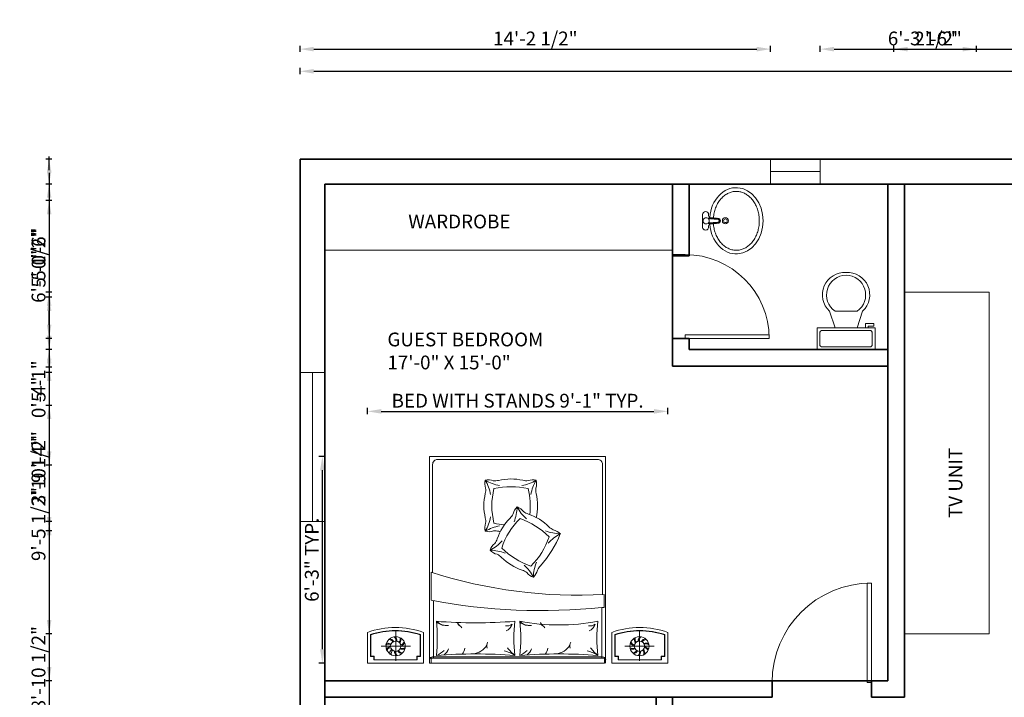
# Model space of a CAD drawing. Units: inches. Extents: x -100 to 766, y -562 to 63.
# Tile 8 of 11: x -100 to 257, y -182 to 63. Entities that reach past the tile are written whole.
import ezdxf

# ---------------------------------------------------------------- set-up
doc = ezdxf.new("R2010")
doc.units = ezdxf.units.IN
for name, color, linetype, lineweight in [('A-ANNO-DIMS', 2, 'Continuous', 18), ('A-ANNO-TEXT', 7, 'Continuous', 18), ('A-AREA-IDEN', 7, 'Continuous', 18), ('A-DOOR', 3, 'Continuous', 18), ('A-FLOR-CASE', 32, 'Continuous', 18), ('A-FLOR-FIXT', 8, 'Continuous', 18), ('A-GLAZ', 4, 'Continuous', 18), ('A-WALL', 7, 'Continuous', 35), ('furn', 8, 'Continuous', 13)]:
    doc.layers.add(name, color=color, linetype=linetype, lineweight=lineweight)
doc.styles.get("Standard").update_dxf_attribs({"font": 'arial.ttf'})
doc.dimstyles.new('ISO-25', dxfattribs={"dimtxt": 5, "dimasz": 5, "dimexe": 1.25, "dimexo": 0.625, "dimtad": 1, "dimlunit": 3, "dimtxsty": 'Standard', "dimcen": 2.5, "dimadec": 0, "dimazin": 0, "dimtfac": 1, "dimtmove": 0, "dimatfit": 3, "dimfxl": 1, "dimfxlon": 1, "dimarcsym": 0})

# ---------------------------------------------------------------- blocks, each defined once
blk = doc.blocks.new('*U2')
for p, q in [((0, 0), (0, -6)), ((40, 0), (40, -6))]:
    blk.add_line(p, q)
blk.add_lwpolyline([(0, 0), (0, 40), (1.75, 40), (1.75, 0)], close=True)
blk.add_arc((0, 0), 40, 0, 90)
blk = doc.blocks.new('*U4')
for p, q in [((9.5, -6), (9.5, -2)), ((-10, -8.5), (-8, -8.5)), ((-10, -9.5), (-10, -8.5)), ((-7, -9.5), (-10, -9.5)), ((-8, -8.5), (-8, -8)), ((-7, -8), (-7, -9.5)), ((-4, -8), (-6, -14)), ((4, -8), (6, -14)), ((4, -14), (-4, -14))]:
    blk.add_line(p, q)
blk.add_lwpolyline([(10.5, -8), (10.5, 0), (-10.5, 0), (-10.5, -8)], close=True)
for points in [[(-9.5, -2), (-9.5, -6)], [(8.5, -1), (-8.5, -1)], [(-8.5, -7), (8.5, -7)]]:
    blk.add_lwpolyline(points)
for centre, radius, start, end in [((-8.625, -1.875), 0.8839, 81.8699, 188.1301), ((8.625, -1.875), 0.8839, 351.8699, 98.1301), ((-8.625, -6.125), 0.8839, 171.869898, 278.1301), ((8.625, -6.125), 0.8839, 261.8699, 8.1301), ((-0.4772, -19.9188), 8.0953, 133.01722, 273.38), ((0.0374, -19.8731), 7.127, 124.50543, 269.7), ((-0.0373, -19.8731), 7.127, 270.3, 55.4946), ((0.4773, -19.9188), 8.0953, 266.62, 46.9828)]:
    blk.add_arc(centre, radius, start, end)
blk = doc.blocks.new('*D9')
at = {"layer": 'A-ANNO-DIMS', "color": 0, "lineweight": -2, "transparency": 16777216}
for p, q in [((1.39, 43.65), (1.39, 45.9)), ((6.39, 44.65), (716.39, 44.65)), ((721.39, 43.65), (721.39, 45.9))]:
    blk.add_line(p, q, dxfattribs=at)
at = {"layer": 'A-ANNO-DIMS', "color": 0, "transparency": 16777216}
for points in [[(6.39, 45.48), (6.39, 43.82), (1.39, 44.65)], [(716.39, 45.48), (716.39, 43.82), (721.39, 44.65)]]:
    blk.add_solid(points, dxfattribs=at)
at = {"layer": 'Defpoints', "color": 0, "transparency": 16777216}
for p in [(721.39, 44.65), (1.39, 12.79), (721.39, 12.79)]:
    blk.add_point(p, dxfattribs=at)
at = {"layer": 'A-ANNO-DIMS', "color": 0, "transparency": 16777216, "insert": (361.39, 47.83), "char_height": 5, "attachment_point": 5}
blk.add_mtext("60'", dxfattribs=at)
blk = doc.blocks.new('A$C359865C9')
for p, q in [((0.26, 0.5858), (0.38, 0.5858)), ((0.26, 0.5258), (0.272, 0.5258)), ((0.368, 0.5258), (0.3809, 0.5258))]:
    blk.add_line(p, q)
for radius in [0.03, 0.018]:
    blk.add_circle((0.3201, 0.3632), radius)
for centre, radius, start, end in [((0.26, 0.5558), 0.03, 90.00613, 270.00613), ((0.32, 0.5495), 0.03, 348.15369, 191.84631), ((0.38, 0.5558), 0.03, 270.00613, 89.98161), ((0.272, 0.5078), 0.018, 0.00613, 90.00613), ((0.32, 0.5495), 0.03, 222.45226, 317.54774), ((0.368, 0.5078), 0.018, 90.00613, 180.00613), ((0.3201, 0.4358), 0.024, 180.00613, 0.00613), ((0.3201, 0.4358), 0.0204, 180.00613, 0.00613), ((0.3201, 0.4358), 0.0144, 180.00613, 0.00613)]:
    blk.add_arc(centre, radius, start, end)
at = {"extrusion": (0, 0, -1)}
blk.add_ellipse((0.3199, 0.5826), major_axis=(-0.00812, 0), ratio=0.392595, dxfattribs=at)
at = {"ltscale": 100, "extrusion": (0, 0, -1)}
blk.add_ellipse((0.3201, 0.258), major_axis=(0.3216, 0), ratio=0.80597, start_param=-1.471508, end_param=4.612925, dxfattribs=at)
for points, knots in [([(0.3475, 0.4801), (0.3477, 0.4801), (0.3479, 0.4801), (0.3648, 0.4788), (0.3813, 0.4763), (0.4136, 0.4692), (0.4293, 0.4645), (0.4593, 0.4531), (0.4737, 0.4464), (0.5006, 0.4312), (0.5131, 0.4227), (0.5361, 0.4042), (0.5465, 0.3942), (0.5649, 0.3732), (0.5729, 0.3622), (0.5864, 0.3393), (0.5918, 0.3275), (0.6, 0.3036), (0.6029, 0.2914), (0.6059, 0.2669), (0.6061, 0.2545), (0.6039, 0.2301), (0.6015, 0.218), (0.5941, 0.1942), (0.5892, 0.1825), (0.5768, 0.1597), (0.5693, 0.1486), (0.552, 0.1275), (0.5422, 0.1174), (0.5203, 0.0986), (0.5083, 0.0899), (0.4825, 0.0741), (0.4686, 0.0671), (0.4396, 0.0549), (0.4243, 0.0498), (0.3929, 0.0418), (0.3767, 0.0388), (0.3439, 0.0352), (0.3273, 0.0344), (0.2942, 0.0353), (0.2776, 0.0369), (0.2452, 0.0422), (0.2293, 0.046), (0.1987, 0.0556), (0.1839, 0.0615), (0.156, 0.0751), (0.1428, 0.0828), (0.1184, 0.0997), (0.1071, 0.109), (0.0869, 0.1288), (0.078, 0.1393), (0.0625, 0.1611), (0.0559, 0.1725), (0.0454, 0.1957), (0.0415, 0.2076), (0.036, 0.2317), (0.0346, 0.2438), (0.0345, 0.2566), (0.0345, 0.2573), (0.0345, 0.258), (0.0345, 0.2664), (0.0351, 0.2749), (0.0382, 0.2956), (0.0413, 0.3078), (0.0502, 0.3317), (0.0559, 0.3434), (0.0699, 0.3661), (0.0782, 0.377), (0.0972, 0.3978), (0.1079, 0.4076), (0.1313, 0.4257), (0.1441, 0.434), (0.1714, 0.4488), (0.186, 0.4553), (0.2163, 0.4662), (0.2321, 0.4706), (0.2628, 0.4769), (0.2776, 0.479), (0.2925, 0.4801)], [1.664851, 1.664851, 1.664851, 1.664851, 1.666804, 1.666804, 1.838807, 1.838807, 2.01081, 2.01081, 2.182814, 2.182814, 2.354817, 2.354817, 2.52682, 2.52682, 2.698824, 2.698824, 2.870827, 2.870827, 3.04283, 3.04283, 3.214834, 3.214834, 3.384783, 3.384783, 3.554732, 3.554732, 3.724681, 3.724681, 3.89463, 3.89463, 4.064578, 4.064578, 4.234527, 4.234527, 4.404476, 4.404476, 4.574425, 4.574425, 4.744374, 4.744374, 4.914323, 4.914323, 5.084272, 5.084272, 5.254221, 5.254221, 5.42417, 5.42417, 5.594119, 5.594119, 5.764068, 5.764068, 5.934016, 5.934016, 6.103965, 6.103965, 6.273914, 6.273914, 6.283185, 6.283185, 6.283185, 6.401959, 6.401959, 6.573962, 6.573962, 6.745965, 6.745965, 6.917969, 6.917969, 7.089972, 7.089972, 7.261975, 7.261975, 7.433979, 7.433979, 7.605982, 7.605982, 7.759676, 7.759676, 7.759676, 7.759676]), ([(0.29, 0.5078), (0.2913, 0.4937), (0.2935, 0.4697), (0.2953, 0.4457), (0.2961, 0.4358)], [0, 0, 0, 0, 35.358253, 60.208758, 60.208758, 60.208758, 60.208758]), ([(0.2907, 0.5434), (0.2946, 0.498), (0.2952, 0.4908), (0.2965, 0.4761), (0.2971, 0.4686), (0.2983, 0.4536), (0.2989, 0.4461), (0.2995, 0.4378), (0.2996, 0.4369), (0.2996, 0.4361)], [2.511178, 2.511178, 2.511178, 2.511178, 20.495008, 20.495008, 39.297594, 39.297594, 58.10018, 58.10018, 60.208758, 60.208758, 60.208758, 60.208758]), ([(0.2979, 0.5293), (0.298, 0.528), (0.2981, 0.5267), (0.2988, 0.5184), (0.2993, 0.5127), (0.3005, 0.4986), (0.301, 0.4933), (0.3014, 0.4884), (0.3015, 0.4875), (0.3017, 0.4857), (0.3017, 0.485), (0.3019, 0.4827), (0.3021, 0.4812), (0.3026, 0.4756), (0.3029, 0.4716), (0.3037, 0.4621), (0.3041, 0.4568), (0.3049, 0.4464), (0.3053, 0.4415), (0.3056, 0.4365)], [4.643985, 4.643985, 4.643985, 4.643985, 5.282102, 5.282102, 8.976667, 8.976667, 16.365798, 16.365798, 18.536065, 18.536065, 20.434607, 20.434607, 24.231692, 24.231692, 34.371999, 34.371999, 47.807513, 47.807513, 60.208758, 60.208758, 60.208758, 60.208758]), ([(0.3422, 0.5293), (0.3421, 0.528), (0.342, 0.5267), (0.3412, 0.5184), (0.3408, 0.5127), (0.3395, 0.4986), (0.3391, 0.4933), (0.3387, 0.4884), (0.3386, 0.4875), (0.3384, 0.4857), (0.3383, 0.485), (0.3381, 0.4827), (0.338, 0.4812), (0.3375, 0.4756), (0.3372, 0.4716), (0.3364, 0.4621), (0.336, 0.4568), (0.3352, 0.4464), (0.3348, 0.4415), (0.3345, 0.4365)], [4.643985, 4.643985, 4.643985, 4.643985, 5.282102, 5.282102, 8.976667, 8.976667, 16.365798, 16.365798, 18.536065, 18.536065, 20.434607, 20.434607, 24.231692, 24.231692, 34.371999, 34.371999, 47.807513, 47.807513, 60.208758, 60.208758, 60.208758, 60.208758]), ([(0.3494, 0.5434), (0.3455, 0.498), (0.3449, 0.4908), (0.3436, 0.4761), (0.343, 0.4686), (0.3418, 0.4536), (0.3412, 0.4461), (0.3406, 0.4378), (0.3405, 0.4369), (0.3404, 0.4361)], [2.511178, 2.511178, 2.511178, 2.511178, 20.495008, 20.495008, 39.297594, 39.297594, 58.10018, 58.10018, 60.208758, 60.208758, 60.208758, 60.208758]), ([(0.35, 0.5078), (0.3487, 0.4937), (0.3466, 0.4697), (0.3448, 0.4457), (0.344, 0.4358)], [0, 0, 0, 0, 35.358253, 60.208758, 60.208758, 60.208758, 60.208758])]:
    blk.add_open_spline(points, degree=3, knots=knots)
blk = doc.blocks.new('WIN-54IN')
blk.add_line((4.5, 54), (4.5, 0))
blk.add_lwpolyline([(0, 54), (9, 54), (9, 0), (0, 0)], close=True)
blk = doc.blocks.new('WIN-18IN')
blk.add_line((4.5, 18), (4.5, 0))
blk.add_lwpolyline([(0, 18), (9, 18), (9, 0), (0, 0)], close=True)
blk = doc.blocks.new('BED-DOUBLE-WITH-NIGHTSTANDS')
for p, q in [((23.96, 1.73), (23.96, 22.55)), ((84.9, 1.73), (84.9, 20.16)), ((10.25, 11.43), (10.25, 0.8)), ((98.58, 11.43), (98.58, 0.79)), ((4.93, 6.11), (15.57, 6.11)), ((103.9, 6.11), (93.26, 6.11)), ((85.22, 2.28), (23.61, 2.28))]:
    blk.add_line(p, q)
for points in [[(86.32, 0), (86.32, 74.89), (22.5, 74.89), (22.5, 0)], [(2.43, 1.11), (2.43, 2.44), (1.11, 2.44)], [(2.32, 1.11), (2.32, 2.32), (1.11, 2.32)], [(2.32, 1.22), (17.97, 1.22)], [(2.32, 1.11), (17.97, 1.11)], [(17.85, 1.11), (17.85, 2.44), (19.18, 2.44)], [(17.97, 1.11), (17.97, 2.32), (19.18, 2.32)], [(23.1, 0), (23.1, 1.73), (85.95, 1.73), (85.95, 0), (22.5, 0)], [(90.97, 1.11), (90.97, 2.44), (89.64, 2.44)], [(90.86, 1.11), (90.86, 2.33), (89.64, 2.33)], [(106.5, 1.22), (90.86, 1.22)], [(106.5, 1.11), (90.86, 1.11)], [(106.39, 1.11), (106.39, 2.44), (107.72, 2.44)], [(106.5, 1.11), (106.5, 2.33), (107.72, 2.33)]]:
    blk.add_lwpolyline(points)
for points in [[(85.22, 24.82), (85.22, 71.94, 0.414214), (83.37, 73.78), (25.45, 73.78, 0.414214), (23.61, 71.94), (23.61, 32.78)], [(42.71, 66.24, 0.159461), (42.84, 63.34, -0.076283), (42.71, 61.4, 0.115075), (42.71, 52.64, -0.076283), (42.84, 50.7, 0.159461), (42.71, 47.8)], [(44.62, 61.06, 0.091296), (42.71, 66.24, 0.091296), (47.89, 64.35)], [(55.97, 64.35, 0.091296), (61.15, 66.24, 0.091296), (59.25, 61.06, 0.091296)], [(58.24, 63.23, 0.111006), (45.84, 63.22, 0.119549), (45.84, 50.66, 0.033212), (49.65, 50.08)], [(54.24, 56.57, 0.159461), (52.81, 54.04, -0.076283), (51.68, 52.46, 0.115075), (47.05, 45.03, -0.076283), (46.13, 43.32, 0.159461), (44.49, 40.92)], [(53.12, 51.17, 0.091296), (54.24, 56.57, 0.091296), (57.64, 52.23)], [(47.89, 49.69, 0.091296), (42.71, 47.8, 0.091296), (44.62, 52.98, 0.091296)], [(65.83, 45.8, 0.111006), (55.29, 52.35, 0.119549), (48.65, 41.69, 0.107813), (59.16, 35.11)], [(64.49, 47.96, 0.091296), (69.89, 46.82, 0.091296), (65.54, 43.43, 0.091296)], [(49.89, 39.78, 0.091296), (44.49, 40.92, 0.091296), (48.84, 44.31, 0.091296)], [(59.21, 35.12, 0.121865), (65.83, 45.8, 0.121865)], [(61.26, 36.57, 0.091296), (60.14, 31.16, 0.091296), (56.74, 35.51, 0.091296)], [(19.18, 2.32), (19.18, 10.3, 0.167087), (1.11, 10.3), (1.11, 2.32)], [(19.07, 2.32), (19.07, 10.22, 0.165559), (1.22, 10.22), (1.22, 2.32)], [(89.64, 2.33), (89.64, 10.3, -0.167087), (107.72, 10.3), (107.72, 2.33)], [(89.75, 2.33), (89.75, 10.22, -0.165559), (107.61, 10.22), (107.61, 2.33)]]:
    blk.add_lwpolyline(points, format="xyb")
for points in [[(85.77, 20.16), (84.9, 20.16, -0.072944), (23.1, 22.73), (23.1, 32.96, 0.092568), (85.77, 24.85)], [(53.41, 15.12, 0.058596), (53.41, 2.79, 0.036648), (24.98, 2.79, 0.052163), (24.98, 15.12, 0.036967)], [(83.49, 15.12, 0.058596), (83.49, 2.79, 0.036889), (55.25, 2.79, 0.052163), (55.25, 15.12, 0.093111)], [(0, 11.07), (0, 0), (20.29, 0), (20.29, 11.07, 0.181818)], [(108.83, 11.07), (108.83, 0), (88.54, 0), (88.54, 11.07, -0.181818)]]:
    blk.add_lwpolyline(points, format="xyb", close=True)
for centre, radius in [((10.25, 6.11), 3.48), ((10.25, 6.11), 1.88), ((98.58, 6.11), 3.48), ((98.58, 6.11), 1.88)]:
    blk.add_circle(centre, radius)
for centre, radius, start, end in [((43.85, 61.01), 5.35, 70.7023, 102.284), ((46.15, 72.45), 6.4, 265.2252, 282.6741), ((51.99, 47.44), 19.27, 77.0576, 103.3153), ((57.67, 72.48), 6.4, 257.6988, 275.1477), ((59.91, 61.73), 4.68, 74.5791, 110.8198), ((56.65, 64.98), 4.68, 339.3666, 15.6073), ((32.87, 56.89), 26.15, 353.1956, 14.0284), ((67.41, 62.78), 6.4, 175.0387, 192.4877), ((42.38, 57.02), 19.27, 346.8711, 13.1289), ((52.44, 51.53), 5.35, 38.7754, 70.3571), ((60.44, 60.02), 6.4, 233.2983, 250.7472), ((52.18, 35.71), 19.27, 45.1307, 71.3884), ((44.09, 51.89), 4.32, 251.3996, 291.5774), ((46.25, 41.5), 6.4, 77.6988, 95.1477), ((51.93, 66.54), 19.27, 257.0576, 258.7033), ((32.5, 62.1), 40.4, 318.3818, 337.7644), ((70.24, 53.96), 6.4, 225.7718, 243.2208), ((66.46, 43.65), 4.68, 42.6522, 78.8929), ((47.82, 43.66), 4.32, 219.4726, 259.6505), ((44.16, 33.7), 6.4, 45.7718, 63.2208), ((62.22, 51.95), 19.27, 225.1307, 251.3884), ((53.96, 27.63), 6.4, 53.2983, 70.7472), ((61.38, 35.5), 4.51, 217.2937, 254.0973), ((56.98, 34.61), 4.68, 312.4658, 348.7065), ((67.28, 30.79), 6.4, 135.5854, 153.0343), ((27.82, 16.88), 3.19, 213.6349, 270.8456), ((28.76, 18.64), 5.04, 224.406, 276.8342), ((33.7, 14.59), 1.03, 173.7543, 257.2187), ((45.1, 23.69), 15.4, 216.2085, 225.0849), ((58.85, 18.64), 5.04, 224.406, 276.8342), ((57.9, 16.88), 3.19, 213.6349, 270.8456), ((63.79, 14.59), 1.03, 173.7543, 257.2187), ((75.18, 23.69), 15.4, 216.2085, 225.0849), ((50.68, 16.26), 2.8, 256.4823, 308.5563), ((48.55, 15.4), 4.1, 294.2916, 340.9896), ((80.77, 16.26), 2.8, 256.4823, 308.5563), ((78.64, 15.4), 4.1, 294.2916, 340.9896), ((7.62, 4.92), 2.23, 69.5103, 115.83), ((7.79, 6.82), 1.7, 31.462, 91.6998), ((7.68, 6.63), 2.23, 33.5103, 79.83), ((8.68, 8.13), 1.7, 355.462, 55.6998), ((8.47, 8.04), 2.23, 357.5103, 43.83), ((10.16, 8.67), 1.7, 319.462, 19.6998), ((9.94, 8.72), 2.23, 321.5103, 7.83), ((11.68, 8.23), 1.7, 283.462, 343.6998), ((11.53, 8.4), 2.23, 285.5103, 331.83), ((46.36, 6.29), 3.06, 155.8927, 196.1192), ((76.44, 6.29), 3.06, 155.8927, 196.1192), ((97.3, 8.4), 2.23, 208.17, 254.4897), ((97.15, 8.23), 1.7, 196.3002, 256.538), ((98.88, 8.72), 2.23, 172.17, 218.4897), ((98.67, 8.67), 1.7, 160.3002, 220.538), ((100.36, 8.04), 2.23, 136.17, 182.4897), ((100.15, 8.13), 1.7, 124.3002, 184.538), ((101.15, 6.63), 2.23, 100.17, 146.4897), ((101.03, 6.82), 1.7, 88.3002, 148.538), ((100.96, 5.02), 2.23, 64.17, 110.4897), ((7.59, 5.14), 1.7, 67.462, 127.6998), ((8.72, 3.73), 2.23, 105.5103, 151.83), ((8.57, 3.9), 1.7, 103.462, 163.6998), ((10.3, 3.42), 2.23, 141.5103, 187.83), ((10.34, 3.56), 1.7, 139.462, 199.6998), ((12.03, 4.19), 2.23, 177.5103, 223.83), ((11.82, 4.1), 1.7, 175.462, 235.6998), ((12.82, 5.6), 2.23, 213.5103, 259.83), ((12.71, 5.41), 1.7, 211.462, 271.6998), ((12.63, 7.21), 2.23, 249.5103, 295.83), ((12.65, 6.99), 1.7, 247.462, 307.6998), ((21.28, 11.24), 9.3, 294.6457, 314.1585), ((24.5, 6.89), 5.16, 310.5354, 340.3558), ((30.57, 6.21), 4.8, 321.8174, 349.8987), ((37.48, 10.1), 6.84, 276.6849, 328.3182), ((46.85, -7.52), 12.22, 57.5379, 77.5233), ((62.65, 14.32), 14.78, 216.4935, 231.2792), ((51.37, 11.24), 9.3, 294.6457, 314.1585), ((54.59, 6.89), 5.16, 310.5354, 340.3558), ((60.65, 6.21), 4.8, 321.8174, 349.8987), ((67.57, 10.1), 6.84, 276.6849, 328.3182), ((76.94, -7.52), 12.22, 57.5379, 77.5233), ((92.74, 14.32), 14.78, 216.4935, 231.2792), ((96.17, 6.99), 1.7, 232.3002, 292.538), ((96.2, 7.21), 2.23, 244.17, 290.4897), ((96.12, 5.41), 1.7, 268.3002, 328.538), ((96.01, 5.6), 2.23, 280.17, 326.4897), ((97, 4.1), 1.7, 304.3002, 4.538), ((96.8, 4.19), 2.23, 316.17, 2.4897), ((98.49, 3.56), 1.7, 340.3002, 40.538), ((98.27, 3.51), 2.23, 352.17, 38.4897), ((100.98, 5.24), 1.7, 52.3002, 112.538), ((100, 3.99), 1.7, 16.3002, 76.538), ((99.86, 3.83), 2.23, 28.17, 74.4897), ((23.61, 1.17), 1.11, 90, 180), ((85.22, 1.17), 1.11, 0, 90)]:
    blk.add_arc(centre, radius, start, end)
blk = doc.blocks.new('*D30')
at = {"layer": 'A-ANNO-DIMS', "color": 0, "lineweight": -2, "transparency": 16777216}
for p, q in [((25.81, -79.59), (25.81, -77.34)), ((134.64, -79.59), (134.64, -77.34)), ((30.81, -78.59), (129.64, -78.59))]:
    blk.add_line(p, q, dxfattribs=at)
at = {"layer": 'A-ANNO-DIMS', "color": 0, "transparency": 16777216}
for points in [[(30.81, -77.76), (30.81, -79.42), (25.81, -78.59)], [(129.64, -77.76), (129.64, -79.42), (134.64, -78.59)]]:
    blk.add_solid(points, dxfattribs=at)
at = {"layer": 'Defpoints', "color": 0, "transparency": 16777216}
for p in [(134.64, -78.59), (25.81, -94.91), (134.64, -94.91)]:
    blk.add_point(p, dxfattribs=at)
at = {"layer": 'A-ANNO-DIMS', "color": 0, "transparency": 16777216, "insert": (80.23, -75.38), "char_height": 5, "attachment_point": 5}
blk.add_mtext('BED WITH STANDS 9\'-1" TYP.', dxfattribs=at)
blk = doc.blocks.new('*D31')
at = {"layer": 'A-ANNO-DIMS', "color": 0, "lineweight": -2, "transparency": 16777216}
for p, q in [((10.49, -94.91), (8.24, -94.91)), ((9.49, -164.8), (9.49, -99.91)), ((10.49, -169.8), (8.24, -169.8))]:
    blk.add_line(p, q, dxfattribs=at)
at = {"layer": 'A-ANNO-DIMS', "color": 0, "transparency": 16777216}
for points in [[(8.66, -99.91), (10.32, -99.91), (9.49, -94.91)], [(8.66, -164.8), (10.32, -164.8), (9.49, -169.8)]]:
    blk.add_solid(points, dxfattribs=at)
at = {"layer": 'Defpoints', "color": 0, "transparency": 16777216}
for p in [(9.49, -94.91), (25.81, -94.91), (25.81, -169.8)]:
    blk.add_point(p, dxfattribs=at)
at = {"layer": 'A-ANNO-DIMS', "color": 0, "transparency": 16777216, "insert": (6.31, -132.36), "char_height": 5, "attachment_point": 5, "rotation": 90}
blk.add_mtext('6\'-3" TYP.', dxfattribs=at)
blk = doc.blocks.new('*D40')
at = {"layer": 'A-ANNO-DIMS', "color": 0, "lineweight": -2, "transparency": 16777216}
for p, q in [((142.39, -557.16), (142.39, -559.41)), ((147.39, -558.16), (209.39, -558.16)), ((214.39, -557.16), (214.39, -559.41))]:
    blk.add_line(p, q, dxfattribs=at)
at = {"layer": 'A-ANNO-DIMS', "color": 0, "transparency": 16777216}
for points in [[(147.39, -557.32), (147.39, -558.99), (142.39, -558.16)], [(209.39, -557.32), (209.39, -558.99), (214.39, -558.16)]]:
    blk.add_solid(points, dxfattribs=at)
at = {"layer": 'Defpoints', "color": 0, "transparency": 16777216}
for p in [(142.39, -56.21), (214.39, -56.21), (214.39, -558.16)]:
    blk.add_point(p, dxfattribs=at)
at = {"layer": 'A-ANNO-DIMS', "color": 0, "transparency": 16777216, "insert": (178.39, -554.98), "char_height": 5, "attachment_point": 5}
blk.add_mtext('6\'-0"', dxfattribs=at)
blk = doc.blocks.new('*D41')
at = {"layer": 'A-ANNO-DIMS', "color": 0, "lineweight": -2, "transparency": 16777216}
for p, q in [((-88.51, 3.79), (-90.76, 3.79)), ((-89.51, -1.21), (-89.51, -51.21)), ((-88.51, -56.21), (-90.76, -56.21))]:
    blk.add_line(p, q, dxfattribs=at)
at = {"layer": 'A-ANNO-DIMS', "color": 0, "transparency": 16777216}
for points in [[(-90.35, -1.21), (-88.68, -1.21), (-89.51, 3.79)], [(-90.35, -51.21), (-88.68, -51.21), (-89.51, -56.21)]]:
    blk.add_solid(points, dxfattribs=at)
at = {"layer": 'Defpoints', "color": 0, "transparency": 16777216}
for p in [(142.39, 3.79), (-89.51, -56.21), (142.39, -56.21)]:
    blk.add_point(p, dxfattribs=at)
at = {"layer": 'A-ANNO-DIMS', "color": 0, "transparency": 16777216, "insert": (-92.69, -26.21), "char_height": 5, "attachment_point": 5, "rotation": 90}
blk.add_mtext('5\'-0"', dxfattribs=at)
blk = doc.blocks.new('*D54')
at = {"layer": 'A-ANNO-DIMS', "color": 0, "lineweight": -2, "transparency": 16777216}
for p, q in [((-88.51, -62.62), (-90.76, -62.62)), ((-89.51, -67.62), (-89.51, -171.21)), ((-88.51, -176.21), (-90.76, -176.21))]:
    blk.add_line(p, q, dxfattribs=at)
at = {"layer": 'A-ANNO-DIMS', "color": 0, "transparency": 16777216}
for points in [[(-90.35, -67.62), (-88.68, -67.62), (-89.51, -62.62)], [(-90.35, -171.21), (-88.68, -171.21), (-89.51, -176.21)]]:
    blk.add_solid(points, dxfattribs=at)
at = {"layer": 'Defpoints', "color": 0, "transparency": 16777216}
for p in [(532.39, -62.62), (-89.51, -176.21), (532.39, -176.21)]:
    blk.add_point(p, dxfattribs=at)
at = {"layer": 'A-ANNO-DIMS', "color": 0, "transparency": 16777216, "insert": (-92.72, -119.41), "char_height": 5, "attachment_point": 5, "rotation": 90}
blk.add_mtext('9\'-5 1/2"', dxfattribs=at)
blk = doc.blocks.new('*D55')
at = {"layer": 'A-ANNO-DIMS', "color": 0, "lineweight": -2, "transparency": 16777216}
for p, q in [((-88.51, -35.41), (-90.76, -35.41)), ((-89.51, -40.41), (-89.51, -154.2)), ((-88.51, -159.2), (-90.76, -159.2))]:
    blk.add_line(p, q, dxfattribs=at)
at = {"layer": 'A-ANNO-DIMS', "color": 0, "transparency": 16777216}
for points in [[(-90.35, -40.41), (-88.68, -40.41), (-89.51, -35.41)], [(-90.35, -154.2), (-88.68, -154.2), (-89.51, -159.2)]]:
    blk.add_solid(points, dxfattribs=at)
at = {"layer": 'Defpoints', "color": 0, "transparency": 16777216}
for p in [(220.39, -35.41), (-89.51, -159.2), (220.39, -159.2)]:
    blk.add_point(p, dxfattribs=at)
at = {"layer": 'A-ANNO-DIMS', "color": 0, "transparency": 16777216, "insert": (-92.69, -97.3), "char_height": 5, "attachment_point": 5, "rotation": 90}
blk.add_mtext('10\'-4"', dxfattribs=at)
blk = doc.blocks.new('*D56')
at = {"layer": 'A-ANNO-DIMS', "color": 0, "lineweight": -2, "transparency": 16777216}
for p, q in [((220.39, -557.16), (220.39, -559.41)), ((225.39, -558.16), (246.11, -558.16)), ((251.11, -557.16), (251.11, -559.41))]:
    blk.add_line(p, q, dxfattribs=at)
at = {"layer": 'A-ANNO-DIMS', "color": 0, "transparency": 16777216}
for points in [[(225.39, -557.32), (225.39, -558.99), (220.39, -558.16)], [(246.11, -557.32), (246.11, -558.99), (251.11, -558.16)]]:
    blk.add_solid(points, dxfattribs=at)
at = {"layer": 'Defpoints', "color": 0, "transparency": 16777216}
for p in [(220.39, -159.2), (251.11, -159.2), (251.11, -558.16)]:
    blk.add_point(p, dxfattribs=at)
at = {"layer": 'A-ANNO-DIMS', "color": 0, "transparency": 16777216, "insert": (235.75, -554.95), "char_height": 5, "attachment_point": 5}
blk.add_mtext('2\'-6 1/2"', dxfattribs=at)
blk = doc.blocks.new('*D57')
at = {"layer": 'A-ANNO-DIMS', "color": 0, "lineweight": -2, "transparency": 16777216}
for p, q in [((1.39, 51.68), (1.39, 53.93)), ((171.91, 51.68), (171.91, 53.93)), ((6.39, 52.68), (166.91, 52.68))]:
    blk.add_line(p, q, dxfattribs=at)
at = {"layer": 'A-ANNO-DIMS', "color": 0, "transparency": 16777216}
for points in [[(6.39, 53.51), (6.39, 51.84), (1.39, 52.68)], [(166.91, 53.51), (166.91, 51.84), (171.91, 52.68)]]:
    blk.add_solid(points, dxfattribs=at)
at = {"layer": 'Defpoints', "color": 0, "transparency": 16777216}
for p in [(171.91, 52.68), (1.39, 12.79), (171.91, 12.79)]:
    blk.add_point(p, dxfattribs=at)
at = {"layer": 'A-ANNO-DIMS', "color": 0, "transparency": 16777216, "insert": (86.65, 55.89), "char_height": 5, "attachment_point": 5}
blk.add_mtext('14\'-2 1/2"', dxfattribs=at)
blk = doc.blocks.new('*D58')
at = {"layer": 'A-ANNO-DIMS', "color": 0, "lineweight": -2, "transparency": 16777216}
for p, q in [((189.91, 51.68), (189.91, 53.93)), ((265.66, 51.68), (265.66, 53.93)), ((194.91, 52.68), (260.66, 52.68))]:
    blk.add_line(p, q, dxfattribs=at)
at = {"layer": 'A-ANNO-DIMS', "color": 0, "transparency": 16777216}
for points in [[(194.91, 53.51), (194.91, 51.84), (189.91, 52.68)], [(260.66, 53.51), (260.66, 51.84), (265.66, 52.68)]]:
    blk.add_solid(points, dxfattribs=at)
at = {"layer": 'Defpoints', "color": 0, "transparency": 16777216}
for p in [(265.66, 52.68), (189.91, 12.79), (265.66, 12.79)]:
    blk.add_point(p, dxfattribs=at)
at = {"layer": 'A-ANNO-DIMS', "color": 0, "transparency": 16777216, "insert": (227.79, 55.89), "char_height": 5, "attachment_point": 5}
blk.add_mtext('6\'-3 1/2"', dxfattribs=at)
blk = doc.blocks.new('*D59')
at = {"layer": 'A-ANNO-DIMS', "color": 0, "lineweight": -2, "transparency": 16777216}
for p, q in [((-88.51, 12.79), (-90.76, 12.79)), ((-89.51, 7.79), (-89.51, -59.48)), ((-88.51, -64.48), (-90.76, -64.48))]:
    blk.add_line(p, q, dxfattribs=at)
at = {"layer": 'A-ANNO-DIMS', "color": 0, "transparency": 16777216}
for points in [[(-90.35, 7.79), (-88.68, 7.79), (-89.51, 12.79)], [(-90.35, -59.48), (-88.68, -59.48), (-89.51, -64.48)]]:
    blk.add_solid(points, dxfattribs=at)
at = {"layer": 'Defpoints', "color": 0, "transparency": 16777216}
for p in [(1.39, 12.79), (-89.51, -64.48), (1.39, -64.48)]:
    blk.add_point(p, dxfattribs=at)
at = {"layer": 'A-ANNO-DIMS', "color": 0, "transparency": 16777216, "insert": (-92.72, -25.85), "char_height": 5, "attachment_point": 5, "rotation": 90}
blk.add_mtext('6\'-5 1/2"', dxfattribs=at)
blk = doc.blocks.new('*D60')
at = {"layer": 'A-ANNO-DIMS', "color": 0, "lineweight": -2, "transparency": 16777216}
for p, q in [((-88.51, -118.48), (-90.76, -118.48)), ((-89.51, -123.48), (-89.51, -219.89)), ((-88.51, -224.89), (-90.76, -224.89))]:
    blk.add_line(p, q, dxfattribs=at)
at = {"layer": 'A-ANNO-DIMS', "color": 0, "transparency": 16777216}
for points in [[(-90.35, -123.48), (-88.68, -123.48), (-89.51, -118.48)], [(-90.35, -219.89), (-88.68, -219.89), (-89.51, -224.89)]]:
    blk.add_solid(points, dxfattribs=at)
at = {"layer": 'Defpoints', "color": 0, "transparency": 16777216}
for p in [(1.39, -118.48), (-89.51, -224.89), (1.39, -224.89)]:
    blk.add_point(p, dxfattribs=at)
at = {"layer": 'A-ANNO-DIMS', "color": 0, "transparency": 16777216, "insert": (-92.72, -171.69), "char_height": 5, "attachment_point": 5, "rotation": 90}
blk.add_mtext('8\'-10 1/2"', dxfattribs=at)
blk = doc.blocks.new('*D75')
at = {"layer": 'A-ANNO-DIMS', "color": 0, "lineweight": -2, "transparency": 16777216}
for p, q in [((-88.51, -37.21), (-90.76, -37.21)), ((-89.51, -42.21), (-89.51, -93.08)), ((-88.51, -98.08), (-90.76, -98.08))]:
    blk.add_line(p, q, dxfattribs=at)
at = {"layer": 'A-ANNO-DIMS', "color": 0, "transparency": 16777216}
for points in [[(-90.35, -42.21), (-88.68, -42.21), (-89.51, -37.21)], [(-90.35, -93.08), (-88.68, -93.08), (-89.51, -98.08)]]:
    blk.add_solid(points, dxfattribs=at)
at = {"layer": 'Defpoints', "color": 0, "transparency": 16777216}
for p in [(620.21, -37.21), (-89.51, -98.08), (620.21, -98.08)]:
    blk.add_point(p, dxfattribs=at)
at = {"layer": 'A-ANNO-DIMS', "color": 0, "transparency": 16777216, "insert": (-92.69, -67.65), "char_height": 5, "attachment_point": 5, "rotation": 90}
blk.add_mtext('5\'-1"', dxfattribs=at)
blk = doc.blocks.new('*D79')
at = {"layer": 'A-ANNO-DIMS', "color": 0, "lineweight": -2, "transparency": 16777216}
for p, q in [((216.52, 51.68), (216.52, 53.93)), ((246.52, 51.68), (246.52, 53.93)), ((221.52, 52.68), (241.52, 52.68))]:
    blk.add_line(p, q, dxfattribs=at)
at = {"layer": 'A-ANNO-DIMS', "color": 0, "transparency": 16777216}
for points in [[(221.52, 53.51), (221.52, 51.84), (216.52, 52.68)], [(241.52, 53.51), (241.52, 51.84), (246.52, 52.68)]]:
    blk.add_solid(points, dxfattribs=at)
at = {"layer": 'Defpoints', "color": 0, "transparency": 16777216}
for p in [(246.52, 52.68), (216.52, -362.21), (246.52, -362.21)]:
    blk.add_point(p, dxfattribs=at)
at = {"layer": 'A-ANNO-DIMS', "color": 0, "transparency": 16777216, "insert": (231.52, 55.86), "char_height": 5, "attachment_point": 5}
blk.add_mtext('2\'-6"', dxfattribs=at)
blk = doc.blocks.new('*D84')
at = {"layer": 'A-ANNO-DIMS', "color": 0, "lineweight": -2, "transparency": 16777216}
for p, q in [((-89.51, 8.79), (-89.51, 13.79)), ((-88.51, 3.79), (-90.76, 3.79)), ((-89.51, 3.79), (-89.51, -2.21)), ((-88.51, -2.21), (-90.76, -2.21)), ((-89.51, -7.21), (-89.51, -26.76))]:
    blk.add_line(p, q, dxfattribs=at)
at = {"layer": 'A-ANNO-DIMS', "color": 0, "transparency": 16777216}
for points in [[(-90.35, 8.79), (-88.68, 8.79), (-89.51, 3.79)], [(-90.35, -7.21), (-88.68, -7.21), (-89.51, -2.21)]]:
    blk.add_solid(points, dxfattribs=at)
at = {"layer": 'Defpoints', "color": 0, "transparency": 16777216}
for p in [(526.39, 3.79), (-89.51, -2.21), (526.39, -2.21)]:
    blk.add_point(p, dxfattribs=at)
at = {"layer": 'A-ANNO-DIMS', "color": 0, "transparency": 16777216, "insert": (-92.69, -19.49), "char_height": 5, "attachment_point": 5, "rotation": 90}
blk.add_mtext('0\'-6"', dxfattribs=at)
blk = doc.blocks.new('*D85')
at = {"layer": 'A-ANNO-DIMS', "color": 0, "lineweight": -2, "transparency": 16777216}
for p, q in [((761.28, -177.21), (761.28, -172.21)), ((760.28, -182.21), (762.53, -182.21)), ((761.28, -182.21), (761.28, -188.21)), ((760.28, -188.21), (762.53, -188.21)), ((761.28, -193.21), (761.28, -212.76))]:
    blk.add_line(p, q, dxfattribs=at)
at = {"layer": 'A-ANNO-DIMS', "color": 0, "transparency": 16777216}
for points in [[(760.45, -177.21), (762.11, -177.21), (761.28, -182.21)], [(760.45, -193.21), (762.11, -193.21), (761.28, -188.21)]]:
    blk.add_solid(points, dxfattribs=at)
at = {"layer": 'Defpoints', "color": 0, "transparency": 16777216}
for p in [(130.39, -182.21), (130.39, -188.21), (761.28, -188.21)]:
    blk.add_point(p, dxfattribs=at)
at = {"layer": 'A-ANNO-DIMS', "color": 0, "transparency": 16777216, "insert": (758.1, -205.49), "char_height": 5, "attachment_point": 5, "rotation": 90}
blk.add_mtext('0\'-6"', dxfattribs=at)
blk = doc.blocks.new('*D86')
at = {"layer": 'A-ANNO-DIMS', "color": 0, "lineweight": -2, "transparency": 16777216}
for p, q in [((-89.51, -47.21), (-89.51, -42.21)), ((-88.51, -52.21), (-90.76, -52.21)), ((-89.51, -52.21), (-89.51, -56.21)), ((-88.51, -56.21), (-90.76, -56.21)), ((-89.51, -61.21), (-89.51, -80.76))]:
    blk.add_line(p, q, dxfattribs=at)
at = {"layer": 'A-ANNO-DIMS', "color": 0, "transparency": 16777216}
for points in [[(-90.35, -47.21), (-88.68, -47.21), (-89.51, -52.21)], [(-90.35, -61.21), (-88.68, -61.21), (-89.51, -56.21)]]:
    blk.add_solid(points, dxfattribs=at)
at = {"layer": 'Defpoints', "color": 0, "transparency": 16777216}
for p in [(142.39, -52.21), (-89.51, -56.21), (142.39, -56.21)]:
    blk.add_point(p, dxfattribs=at)
at = {"layer": 'A-ANNO-DIMS', "color": 0, "transparency": 16777216, "insert": (-92.69, -73.49), "char_height": 5, "attachment_point": 5, "rotation": 90}
blk.add_mtext('0\'-4"', dxfattribs=at)
blk = doc.blocks.new('*D88')
at = {"layer": 'A-ANNO-DIMS', "color": 0, "lineweight": -2, "transparency": 16777216}
for p, q in [((-88.51, -76.41), (-90.76, -76.41)), ((-89.51, -81.41), (-89.51, -116.91)), ((-88.51, -121.91), (-90.76, -121.91))]:
    blk.add_line(p, q, dxfattribs=at)
at = {"layer": 'A-ANNO-DIMS', "color": 0, "transparency": 16777216}
for points in [[(-90.35, -81.41), (-88.68, -81.41), (-89.51, -76.41)], [(-90.35, -116.91), (-88.68, -116.91), (-89.51, -121.91)]]:
    blk.add_solid(points, dxfattribs=at)
at = {"layer": 'Defpoints', "color": 0, "transparency": 16777216}
for p in [(310.41, -76.41), (-89.51, -121.91), (310.41, -121.91)]:
    blk.add_point(p, dxfattribs=at)
at = {"layer": 'A-ANNO-DIMS', "color": 0, "transparency": 16777216, "insert": (-92.73, -99.16), "char_height": 5, "attachment_point": 5, "rotation": 90}
blk.add_mtext('3\'-9 1/2"', dxfattribs=at)

msp = doc.modelspace()

# ---------------------------------------------------------------- linework, layer by layer
at = {"layer": 'A-FLOR-CASE'}
msp.add_line((10.388, -20.214), (136.388, -20.214), dxfattribs=at)
msp.add_lwpolyline([(220.388, -35.408), (251.108, -35.408), (251.108, -159.197), (220.388, -159.197)], close=True, dxfattribs=at)
at = {"layer": 'A-WALL'}
for p, q in [((10.388, 3.786), (229.388, 3.786)), ((10.388, -458.214), (10.388, 3.786)), ((136.388, 3.786), (136.388, -56.214)), ((142.388, 3.786), (142.388, -22.214)), ((214.388, 3.786), (214.388, -176.214)), ((220.388, 3.786), (220.388, -182.214)), ((220.388, -182.214), (220.388, 3.786)), ((229.388, 3.786), (271.388, 3.786)), ((142.388, -22.214), (136.388, -22.214)), ((142.388, -52.214), (136.388, -52.214)), ((142.388, -52.214), (142.388, -56.214)), ((136.388, -56.214), (136.388, -62.214)), ((142.388, -56.214), (214.388, -56.214)), ((136.388, -62.214), (180.388, -62.214)), ((180.388, -62.214), (212.388, -62.214)), ((210.388, -62.214), (214.388, -62.214)), ((214.388, -176.214), (10.388, -176.214)), ((172.434, -176.214), (172.434, -182.214)), ((208.434, -176.214), (208.434, -182.214)), ((172.434, -182.214), (10.388, -182.214)), ((130.388, -188.214), (130.388, -182.214)), ((136.388, -272.214), (136.388, -182.214)), ((214.388, -182.214), (208.434, -182.214)), ((211.351, -182.214), (220.388, -182.214))]:
    msp.add_line(p, q, dxfattribs=at)
msp.add_lwpolyline([(1.388, 12.786), (721.388, 12.786), (721.388, -467.214), (1.388, -467.214)], close=True, dxfattribs=at)

# ---------------------------------------------------------------- block references
at = {"layer": 'A-DOOR', "xscale": -0.7609430435882376, "yscale": 0.7609430435882376, "zscale": 0.7609430435882376, "rotation": 270}
msp.add_blockref('*U2', (140.953, -52.214), dxfattribs=at)
at = {"layer": 'A-DOOR', "xscale": -0.900419896884199, "yscale": 0.900419896884199, "zscale": 0.900419896884199}
msp.add_blockref('*U2', (208.434, -176.812), dxfattribs=at)
at = {"layer": 'A-FLOR-FIXT', "xscale": 37.38131337077302, "yscale": 37.38131337077302, "zscale": 37.38131337077302, "rotation": 90}
msp.add_blockref('A$C359865C9', (169.117, -21.502), dxfattribs=at)
at = {"layer": 'A-FLOR-FIXT', "rotation": 180}
msp.add_blockref('*U4', (199.262, -56.264), dxfattribs=at)
at = {"layer": 'A-GLAZ', "rotation": 270.0000000000001}
msp.add_blockref('WIN-18IN', (171.913, 12.785), dxfattribs=at)
at = {"layer": 'A-GLAZ'}
msp.add_blockref('WIN-54IN', (1.388, -118.484), dxfattribs=at)
at = {"layer": 'furn'}
msp.add_blockref('BED-DOUBLE-WITH-NIGHTSTANDS', (25.814, -169.801), dxfattribs=at)

# ---------------------------------------------------------------- texts
at = {"layer": 'A-ANNO-TEXT', "insert": (40.608, -7.299), "char_height": 5, "attachment_point": 1}
msp.add_mtext_dynamic_manual_height_columns('WARDROBE', width=41.4154, gutter_width=12.5, heights=[0], dxfattribs=at)
at = {"layer": 'A-ANNO-TEXT', "insert": (236.407, -117.249), "char_height": 5, "attachment_point": 1, "rotation": 90}
msp.add_mtext_dynamic_manual_height_columns('TV UNIT', width=119.92154, gutter_width=12.5, heights=[0], dxfattribs=at)
at = {"layer": 'A-AREA-IDEN', "insert": (33.054, -50.034), "char_height": 5, "attachment_point": 1}
msp.add_mtext_dynamic_manual_height_columns('GUEST BEDROOM\\P17\'-0" X 15\'-0"', width=95.79153, gutter_width=12.5, heights=[0], dxfattribs=at)

# ---------------------------------------------------------------- dimensions: what is measured, and where the dimension line sits
at = {"layer": 'A-ANNO-DIMS'}
for base, p1, p2, override, picture, middle in [((171.914, 52.678), (1.388, 12.786), (171.914, 12.786), {"dimdec": 1, "dimlfac": 1, "dimrnd": 0, "dimzin": 1, "dimdsep": 46, "dimlunit": 4, "dimfrac": 2}, '*D57', (86.651, 55.888)), ((265.66, 52.678), (189.914, 12.786), (265.66, 12.786), {"dimdec": 1, "dimlfac": 1, "dimrnd": 0, "dimzin": 1, "dimdsep": 46, "dimlunit": 4, "dimfrac": 2}, '*D58', (227.787, 55.89)), ((246.522, 52.678), (216.522, -362.214), (246.522, -362.214), {"dimdec": 1, "dimlfac": 1, "dimrnd": 0, "dimzin": 1, "dimdsep": 46, "dimlunit": 4, "dimfrac": 2}, '*D79', (231.522, 55.855)), ((721.388, 44.65), (1.388, 12.786), (721.388, 12.786), {"dimclrd": 0, "dimclre": 0, "dimclrt": 0}, '*D9', (361.388, 47.828)), ((214.388, -558.156), (142.388, -56.214), (214.388, -56.214), {"dimdec": 1, "dimlfac": 1, "dimrnd": 0, "dimzin": 1, "dimdsep": 46, "dimlunit": 4, "dimfrac": 2}, '*D40', (178.388, -554.979)), ((251.108, -558.156), (220.388, -159.197), (251.108, -159.197), {"dimdec": 1, "dimlfac": 1, "dimrnd": 0, "dimzin": 1, "dimdsep": 46, "dimlunit": 4, "dimfrac": 2}, '*D56', (235.748, -554.946))]:
    dim = msp.add_linear_dim(base=base, p1=p1, p2=p2, dimstyle='ISO-25', override=override, dxfattribs=at)
    dim.commit()
    dim.dimension.update_dxf_attribs({"geometry": picture, "text_midpoint": middle})
for base, p1, p2, picture, middle in [((-89.513, -64.484), (1.388, 12.786), (1.388, -64.484), '*D59', (-92.723, -25.849)), ((-89.513, -2.214), (526.388, 3.786), (526.388, -2.214), '*D84', (-92.691, -19.485)), ((-89.513, -56.214), (142.388, 3.786), (142.388, -56.214), '*D41', (-92.691, -26.214)), ((-89.513, -159.197), (220.388, -35.408), (220.388, -159.197), '*D55', (-92.691, -97.302)), ((-89.513, -98.077), (620.215, -37.214), (620.215, -98.077), '*D75', (-92.691, -67.645)), ((-89.513, -56.214), (142.388, -52.214), (142.388, -56.214), '*D86', (-92.691, -73.485)), ((-89.513, -176.214), (532.388, -62.615), (532.388, -176.214), '*D54', (-92.723, -119.415)), ((-89.513, -121.911), (310.414, -76.409), (310.414, -121.911), '*D88', (-92.725, -99.16)), ((-89.513, -224.892), (1.388, -118.484), (1.388, -224.892), '*D60', (-92.723, -171.688)), ((761.28, -188.214), (130.388, -182.214), (130.388, -188.214), '*D85', (758.102, -205.485))]:
    dim = msp.add_linear_dim(base=base, p1=p1, p2=p2, angle=90, dimstyle='ISO-25', override={"dimdec": 1, "dimlfac": 1, "dimrnd": 0, "dimzin": 1, "dimdsep": 46, "dimlunit": 4, "dimfrac": 2}, dxfattribs=at)
    dim.commit()
    dim.dimension.update_dxf_attribs({"geometry": picture, "text_midpoint": middle})
dim = msp.add_linear_dim(base=(134.64, -78.59), p1=(25.814, -94.914), p2=(134.64, -94.914), text='BED WITH STANDS <> TYP.', dimstyle='ISO-25', override={"dimdec": 1, "dimlfac": 1, "dimrnd": 0, "dimzin": 1, "dimdsep": 46, "dimlunit": 4, "dimfrac": 2}, dxfattribs=at)
dim.commit()
dim.dimension.update_dxf_attribs({"geometry": '*D30', "text_midpoint": (80.227, -75.38)})
dim = msp.add_linear_dim(base=(9.49, -94.914), p1=(25.814, -169.801), p2=(25.814, -94.914), angle=90, text='<> TYP.', dimstyle='ISO-25', override={"dimdec": 1, "dimlfac": 1, "dimrnd": 0, "dimzin": 1, "dimdsep": 46, "dimlunit": 4, "dimfrac": 2}, dxfattribs=at)
dim.commit()
dim.dimension.update_dxf_attribs({"geometry": '*D31', "text_midpoint": (6.311, -132.358)})

doc.saveas('drawing.dxf')
